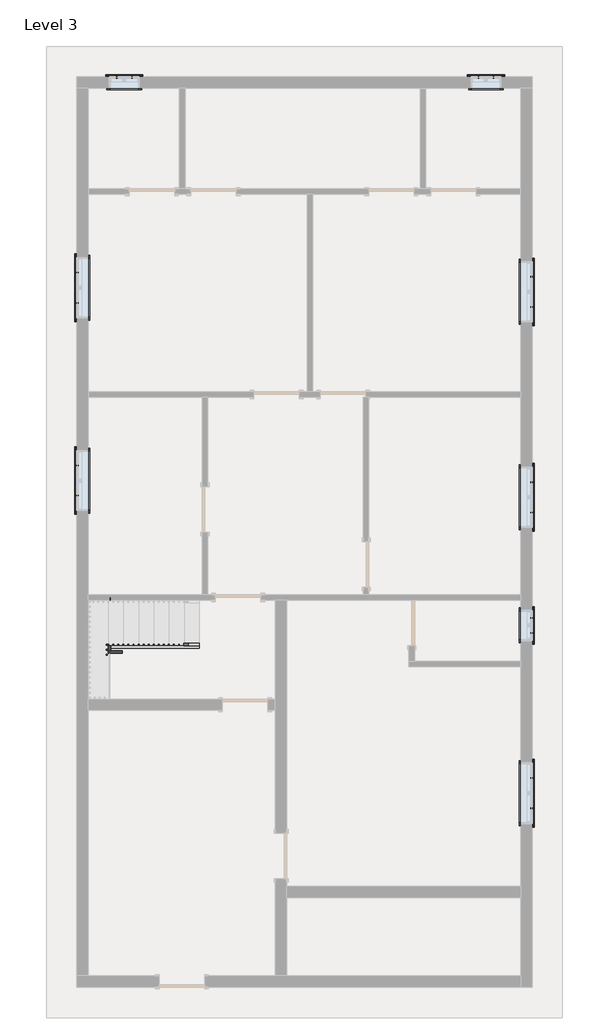
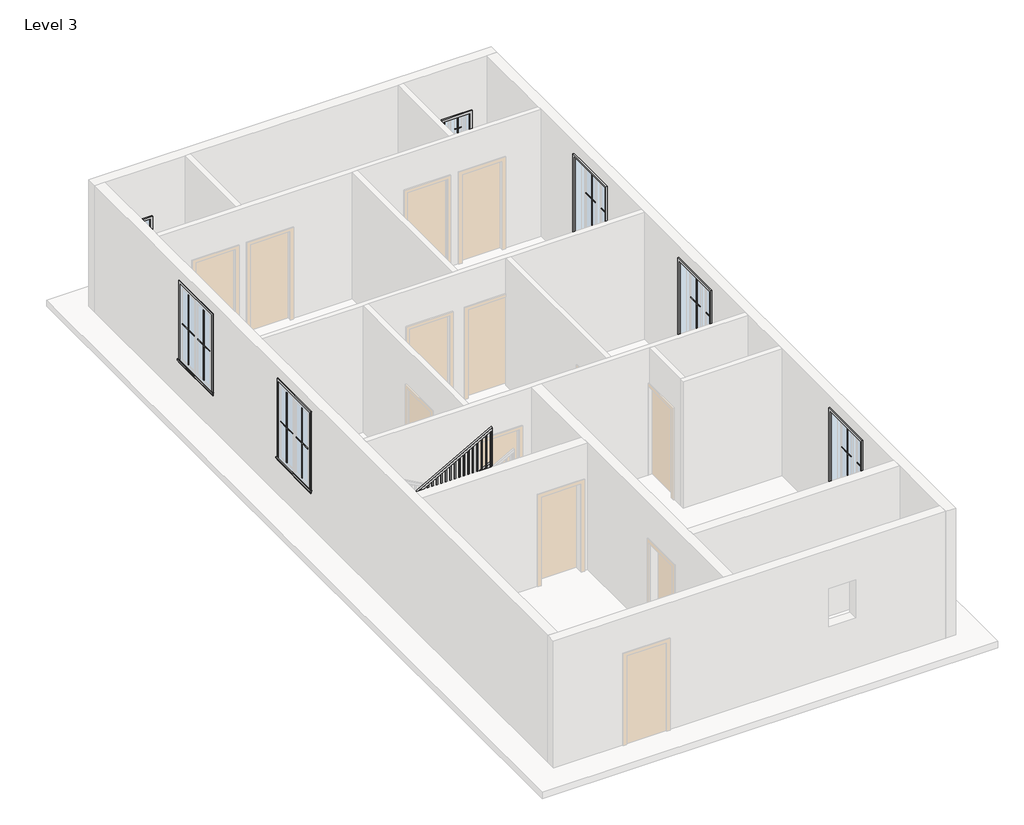
# One storey, part 3 of 3: 32 proxies, 6 members, 1 railing.
"""IFC4 building model written with IfcOpenShell, lengths in millimetres."""

from ifc_helpers import new_model, si_unit, frame, origin, place, context, project, spatial, polyline, outline, extrude, faceted_brep, transform, mapped, element, save
from components import muntin_pattern_2x2_muntin_pattern_2x2_2b4d9f72, muntin_pattern_2x2_muntin_pattern_2x2_ef995ed3, muntin_pattern_2x2_muntin_pattern_2x2_53152e2c, muntin_pattern_2x2_muntin_pattern_2x2_e8f3e573, trim_window_exterior_flat_with_sill_b7e4d11c, trim_window_exterior_flat_with_sill_a665a915, trim_window_interior_flat_picture_frame_936b8d2a, trim_window_interior_flat_picture_frame_d485c387

model = new_model("IFC4")

# Units and contexts
model_context = context("Model", 3, world=origin())
ifc_project = project(units=[si_unit("LENGTHUNIT", "METRE", prefix="MILLI")], contexts=[model_context])

# Site, building, storey
site = spatial("IfcSite", under=ifc_project)
building = spatial("IfcBuilding", under=site)
storey = spatial("IfcBuildingStorey", under=building, Name="Level 3", Elevation=6096.0)

# Proxies
placement = place(None, origin())
muntin_pattern_2x2_muntin_pattern_2x2_shape = muntin_pattern_2x2_muntin_pattern_2x2_2b4d9f72(model_context)
element("IfcBuildingElementProxy", 1, Name="Muntin Pattern_2x2 : Muntin Pattern_2x2", ObjectType="Muntin Pattern_2x2 : Muntin Pattern_2x2", at=placement, inside=storey, context=model_context, shape_type="MappedRepresentation", body=[
    mapped(muntin_pattern_2x2_muntin_pattern_2x2_shape, transform((1279.525, 5811.8375, 7080.25), x_axis=(0.0, 1.0, 0.0), y_axis=(-1.0, 0.0, 0.0), z_axis=(0.0, 0.0, 1.0))),
])
element("IfcBuildingElementProxy", 2, Name="Muntin Pattern_2x2 : Muntin Pattern_2x2", ObjectType="Muntin Pattern_2x2 : Muntin Pattern_2x2", at=placement, inside=storey, context=model_context, shape_type="MappedRepresentation", body=[
    mapped(muntin_pattern_2x2_muntin_pattern_2x2_shape, transform((1279.525, 9685.3375, 7080.25), x_axis=(0.0, 1.0, 0.0), y_axis=(-1.0, 0.0, 0.0), z_axis=(0.0, 0.0, 1.0))),
])
element("IfcBuildingElementProxy", 3, Name="Muntin Pattern_2x2 : Muntin Pattern_2x2", ObjectType="Muntin Pattern_2x2 : Muntin Pattern_2x2", at=placement, inside=storey, context=model_context, shape_type="MappedRepresentation", body=[
    mapped(muntin_pattern_2x2_muntin_pattern_2x2_shape, transform((10404.475, 10209.2125, 7080.25), x_axis=(0.0, -1.0, 0.0), y_axis=(1.0, 0.0, 0.0), z_axis=(0.0, 0.0, 1.0))),
])
element("IfcBuildingElementProxy", 4, Name="Muntin Pattern_2x2 : Muntin Pattern_2x2", ObjectType="Muntin Pattern_2x2 : Muntin Pattern_2x2", at=placement, inside=storey, context=model_context, shape_type="MappedRepresentation", body=[
    mapped(muntin_pattern_2x2_muntin_pattern_2x2_shape, transform((10404.475, 6081.7125, 7080.25), x_axis=(0.0, -1.0, 0.0), y_axis=(1.0, 0.0, 0.0), z_axis=(0.0, 0.0, 1.0))),
])
element("IfcBuildingElementProxy", 5, Name="Muntin Pattern_2x2 : Muntin Pattern_2x2", ObjectType="Muntin Pattern_2x2 : Muntin Pattern_2x2", at=placement, inside=storey, context=model_context, shape_type="MappedRepresentation", body=[
    mapped(muntin_pattern_2x2_muntin_pattern_2x2_shape, transform((10404.475, 138.1125, 7080.25), x_axis=(0.0, -1.0, 0.0), y_axis=(1.0, 0.0, 0.0), z_axis=(0.0, 0.0, 1.0))),
])
muntin_pattern_2x2_muntin_pattern_2x2_2_shape = muntin_pattern_2x2_muntin_pattern_2x2_ef995ed3(model_context)
element("IfcBuildingElementProxy", 6, Name="Muntin Pattern_2x2 : Muntin Pattern_2x2", ObjectType="Muntin Pattern_2x2 : Muntin Pattern_2x2", at=placement, inside=storey, context=model_context, shape_type="MappedRepresentation", body=[
    mapped(muntin_pattern_2x2_muntin_pattern_2x2_2_shape, transform((1279.525, 6418.2625, 7080.25), x_axis=(0.0, -1.0, 0.0), y_axis=(1.0, 0.0, 0.0), z_axis=(0.0, 0.0, 1.0))),
])
element("IfcBuildingElementProxy", 7, Name="Muntin Pattern_2x2 : Muntin Pattern_2x2", ObjectType="Muntin Pattern_2x2 : Muntin Pattern_2x2", at=placement, inside=storey, context=model_context, shape_type="MappedRepresentation", body=[
    mapped(muntin_pattern_2x2_muntin_pattern_2x2_2_shape, transform((1279.525, 10291.7625, 7080.25), x_axis=(0.0, -1.0, 0.0), y_axis=(1.0, 0.0, 0.0), z_axis=(0.0, 0.0, 1.0))),
])
element("IfcBuildingElementProxy", 8, Name="Muntin Pattern_2x2 : Muntin Pattern_2x2", ObjectType="Muntin Pattern_2x2 : Muntin Pattern_2x2", at=placement, inside=storey, context=model_context, shape_type="MappedRepresentation", body=[
    mapped(muntin_pattern_2x2_muntin_pattern_2x2_2_shape, transform((10404.475, 9602.7875, 7080.25), x_axis=(0.0, 1.0, 0.0), y_axis=(-1.0, 0.0, 0.0), z_axis=(0.0, 0.0, 1.0))),
])
element("IfcBuildingElementProxy", 9, Name="Muntin Pattern_2x2 : Muntin Pattern_2x2", ObjectType="Muntin Pattern_2x2 : Muntin Pattern_2x2", at=placement, inside=storey, context=model_context, shape_type="MappedRepresentation", body=[
    mapped(muntin_pattern_2x2_muntin_pattern_2x2_2_shape, transform((10404.475, 5475.2875, 7080.25), x_axis=(0.0, 1.0, 0.0), y_axis=(-1.0, 0.0, 0.0), z_axis=(0.0, 0.0, 1.0))),
])
element("IfcBuildingElementProxy", 10, Name="Muntin Pattern_2x2 : Muntin Pattern_2x2", ObjectType="Muntin Pattern_2x2 : Muntin Pattern_2x2", at=placement, inside=storey, context=model_context, shape_type="MappedRepresentation", body=[
    mapped(muntin_pattern_2x2_muntin_pattern_2x2_2_shape, transform((10404.475, -468.3125, 7080.25), x_axis=(0.0, 1.0, 0.0), y_axis=(-1.0, 0.0, 0.0), z_axis=(0.0, 0.0, 1.0))),
])
muntin_pattern_2x2_muntin_pattern_2x2_3_shape = muntin_pattern_2x2_muntin_pattern_2x2_53152e2c(model_context)
element("IfcBuildingElementProxy", 11, Name="Muntin Pattern_2x2 : Muntin Pattern_2x2", ObjectType="Muntin Pattern_2x2 : Muntin Pattern_2x2", at=placement, inside=storey, context=model_context, shape_type="MappedRepresentation", body=[
    mapped(muntin_pattern_2x2_muntin_pattern_2x2_3_shape, transform((10404.475, 3357.5625, 7080.25), x_axis=(0.0, -1.0, 0.0), y_axis=(1.0, 0.0, 0.0), z_axis=(0.0, 0.0, 1.0))),
])
element("IfcBuildingElementProxy", 12, Name="Muntin Pattern_2x2 : Muntin Pattern_2x2", ObjectType="Muntin Pattern_2x2 : Muntin Pattern_2x2", at=placement, inside=storey, context=model_context, shape_type="MappedRepresentation", body=[
    mapped(muntin_pattern_2x2_muntin_pattern_2x2_3_shape, transform((9336.0875, 14214.475, 7080.25), x_axis=(1.0, 0.0, 0.0), y_axis=(0.0, 1.0, 0.0), z_axis=(0.0, 0.0, 1.0))),
])
element("IfcBuildingElementProxy", 13, Name="Muntin Pattern_2x2 : Muntin Pattern_2x2", ObjectType="Muntin Pattern_2x2 : Muntin Pattern_2x2", at=placement, inside=storey, context=model_context, shape_type="MappedRepresentation", body=[
    mapped(muntin_pattern_2x2_muntin_pattern_2x2_3_shape, transform((2071.6875, 14214.475, 7080.25), x_axis=(1.0, 0.0, 0.0), y_axis=(0.0, 1.0, 0.0), z_axis=(0.0, 0.0, 1.0))),
])
muntin_pattern_2x2_muntin_pattern_2x2_4_shape = muntin_pattern_2x2_muntin_pattern_2x2_e8f3e573(model_context)
element("IfcBuildingElementProxy", 14, Name="Muntin Pattern_2x2 : Muntin Pattern_2x2", ObjectType="Muntin Pattern_2x2 : Muntin Pattern_2x2", at=placement, inside=storey, context=model_context, shape_type="MappedRepresentation", body=[
    mapped(muntin_pattern_2x2_muntin_pattern_2x2_4_shape, transform((10404.475, 3055.9375, 7080.25), x_axis=(0.0, 1.0, 0.0), y_axis=(-1.0, 0.0, 0.0), z_axis=(0.0, 0.0, 1.0))),
])
element("IfcBuildingElementProxy", 15, Name="Muntin Pattern_2x2 : Muntin Pattern_2x2", ObjectType="Muntin Pattern_2x2 : Muntin Pattern_2x2", at=placement, inside=storey, context=model_context, shape_type="MappedRepresentation", body=[
    mapped(muntin_pattern_2x2_muntin_pattern_2x2_4_shape, transform((9637.7125, 14214.475, 7080.25), x_axis=(-1.0, 0.0, 0.0), y_axis=(0.0, -1.0, 0.0), z_axis=(0.0, 0.0, 1.0))),
])
element("IfcBuildingElementProxy", 16, Name="Muntin Pattern_2x2 : Muntin Pattern_2x2", ObjectType="Muntin Pattern_2x2 : Muntin Pattern_2x2", at=placement, inside=storey, context=model_context, shape_type="MappedRepresentation", body=[
    mapped(muntin_pattern_2x2_muntin_pattern_2x2_4_shape, transform((2373.3125, 14214.475, 7080.25), x_axis=(-1.0, 0.0, 0.0), y_axis=(0.0, -1.0, 0.0), z_axis=(0.0, 0.0, 1.0))),
])
trim_window_exterior_flat_with_sill_shape = trim_window_exterior_flat_with_sill_b7e4d11c(model_context)
element("IfcBuildingElementProxy", 17, Name="Trim-Window-Exterior-Flat : with Sill", ObjectType="Trim-Window-Exterior-Flat : with Sill", at=placement, inside=storey, context=model_context, shape_type="MappedRepresentation", body=[
    mapped(trim_window_exterior_flat_with_sill_shape, transform((1270.0, 6115.05, 8839.2), x_axis=(0.0, -1.0, 0.0), y_axis=(0.0, 0.0, 1.0), z_axis=(-1.0, 0.0, 0.0))),
])
element("IfcBuildingElementProxy", 18, Name="Trim-Window-Exterior-Flat : with Sill", ObjectType="Trim-Window-Exterior-Flat : with Sill", at=placement, inside=storey, context=model_context, shape_type="MappedRepresentation", body=[
    mapped(trim_window_exterior_flat_with_sill_shape, transform((1270.0, 9988.55, 8839.2), x_axis=(0.0, -1.0, 0.0), y_axis=(0.0, 0.0, 1.0), z_axis=(-1.0, 0.0, 0.0))),
])
element("IfcBuildingElementProxy", 19, Name="Trim-Window-Exterior-Flat : with Sill", ObjectType="Trim-Window-Exterior-Flat : with Sill", at=placement, inside=storey, context=model_context, shape_type="MappedRepresentation", body=[
    mapped(trim_window_exterior_flat_with_sill_shape, transform((10414.0, 9906.0, 8839.2), x_axis=(0.0, 1.0, 0.0), y_axis=(0.0, 0.0, 1.0), z_axis=(1.0, 0.0, 0.0))),
])
element("IfcBuildingElementProxy", 20, Name="Trim-Window-Exterior-Flat : with Sill", ObjectType="Trim-Window-Exterior-Flat : with Sill", at=placement, inside=storey, context=model_context, shape_type="MappedRepresentation", body=[
    mapped(trim_window_exterior_flat_with_sill_shape, transform((10414.0, 5778.5, 8839.2), x_axis=(0.0, 1.0, 0.0), y_axis=(0.0, 0.0, 1.0), z_axis=(1.0, 0.0, 0.0))),
])
element("IfcBuildingElementProxy", 21, Name="Trim-Window-Exterior-Flat : with Sill", ObjectType="Trim-Window-Exterior-Flat : with Sill", at=placement, inside=storey, context=model_context, shape_type="MappedRepresentation", body=[
    mapped(trim_window_exterior_flat_with_sill_shape, transform((10414.0, -165.1, 8839.2), x_axis=(0.0, 1.0, 0.0), y_axis=(0.0, 0.0, 1.0), z_axis=(1.0, 0.0, 0.0))),
])
trim_window_exterior_flat_with_sill_2_shape = trim_window_exterior_flat_with_sill_a665a915(model_context)
element("IfcBuildingElementProxy", 22, Name="Trim-Window-Exterior-Flat : with Sill", ObjectType="Trim-Window-Exterior-Flat : with Sill", at=placement, inside=storey, context=model_context, shape_type="MappedRepresentation", body=[
    mapped(trim_window_exterior_flat_with_sill_2_shape, transform((10414.0, 3206.75, 7924.8), x_axis=(0.0, 1.0, 0.0), y_axis=(0.0, 0.0, 1.0), z_axis=(1.0, 0.0, 0.0))),
])
element("IfcBuildingElementProxy", 23, Name="Trim-Window-Exterior-Flat : with Sill", ObjectType="Trim-Window-Exterior-Flat : with Sill", at=placement, inside=storey, context=model_context, shape_type="MappedRepresentation", body=[
    mapped(trim_window_exterior_flat_with_sill_2_shape, transform((9486.9, 14224.0, 7924.8), x_axis=(-1.0, 0.0, 0.0), y_axis=(0.0, 0.0, 1.0), z_axis=(0.0, 1.0, 0.0))),
])
element("IfcBuildingElementProxy", 24, Name="Trim-Window-Exterior-Flat : with Sill", ObjectType="Trim-Window-Exterior-Flat : with Sill", at=placement, inside=storey, context=model_context, shape_type="MappedRepresentation", body=[
    mapped(trim_window_exterior_flat_with_sill_2_shape, transform((2222.5, 14224.0, 7924.8), x_axis=(-1.0, 0.0, 0.0), y_axis=(0.0, 0.0, 1.0), z_axis=(0.0, 1.0, 0.0))),
])
trim_window_interior_flat_picture_frame_shape = trim_window_interior_flat_picture_frame_936b8d2a(model_context)
element("IfcBuildingElementProxy", 25, Name="Trim-Window-Interior-Flat : Picture Frame", ObjectType="Trim-Window-Interior-Flat : Picture Frame", at=placement, inside=storey, context=model_context, shape_type="MappedRepresentation", body=[
    mapped(trim_window_interior_flat_picture_frame_shape, transform((1498.6, 6115.05, 8839.2), x_axis=(0.0, 1.0, 0.0), y_axis=(0.0, 0.0, 1.0), z_axis=(1.0, 0.0, 0.0))),
])
element("IfcBuildingElementProxy", 26, Name="Trim-Window-Interior-Flat : Picture Frame", ObjectType="Trim-Window-Interior-Flat : Picture Frame", at=placement, inside=storey, context=model_context, shape_type="MappedRepresentation", body=[
    mapped(trim_window_interior_flat_picture_frame_shape, transform((1498.6, 9988.55, 8839.2), x_axis=(0.0, 1.0, 0.0), y_axis=(0.0, 0.0, 1.0), z_axis=(1.0, 0.0, 0.0))),
])
element("IfcBuildingElementProxy", 27, Name="Trim-Window-Interior-Flat : Picture Frame", ObjectType="Trim-Window-Interior-Flat : Picture Frame", at=placement, inside=storey, context=model_context, shape_type="MappedRepresentation", body=[
    mapped(trim_window_interior_flat_picture_frame_shape, transform((10185.4, 9906.0, 8839.2), x_axis=(0.0, -1.0, 0.0), y_axis=(0.0, 0.0, 1.0), z_axis=(-1.0, 0.0, 0.0))),
])
element("IfcBuildingElementProxy", 28, Name="Trim-Window-Interior-Flat : Picture Frame", ObjectType="Trim-Window-Interior-Flat : Picture Frame", at=placement, inside=storey, context=model_context, shape_type="MappedRepresentation", body=[
    mapped(trim_window_interior_flat_picture_frame_shape, transform((10185.4, 5778.5, 8839.2), x_axis=(0.0, -1.0, 0.0), y_axis=(0.0, 0.0, 1.0), z_axis=(-1.0, 0.0, 0.0))),
])
element("IfcBuildingElementProxy", 29, Name="Trim-Window-Interior-Flat : Picture Frame", ObjectType="Trim-Window-Interior-Flat : Picture Frame", at=placement, inside=storey, context=model_context, shape_type="MappedRepresentation", body=[
    mapped(trim_window_interior_flat_picture_frame_shape, transform((10185.4, -165.1, 8839.2), x_axis=(0.0, -1.0, 0.0), y_axis=(0.0, 0.0, 1.0), z_axis=(-1.0, 0.0, 0.0))),
])
trim_window_interior_flat_picture_frame_2_shape = trim_window_interior_flat_picture_frame_d485c387(model_context)
element("IfcBuildingElementProxy", 30, Name="Trim-Window-Interior-Flat : Picture Frame", ObjectType="Trim-Window-Interior-Flat : Picture Frame", at=placement, inside=storey, context=model_context, shape_type="MappedRepresentation", body=[
    mapped(trim_window_interior_flat_picture_frame_2_shape, transform((10185.4, 3206.75, 7924.8), x_axis=(0.0, -1.0, 0.0), y_axis=(0.0, 0.0, 1.0), z_axis=(-1.0, 0.0, 0.0))),
])
element("IfcBuildingElementProxy", 31, Name="Trim-Window-Interior-Flat : Picture Frame", ObjectType="Trim-Window-Interior-Flat : Picture Frame", at=placement, inside=storey, context=model_context, shape_type="MappedRepresentation", body=[
    mapped(trim_window_interior_flat_picture_frame_2_shape, transform((9486.9, 13995.4, 7924.8), x_axis=(1.0, 0.0, 0.0), y_axis=(0.0, 0.0, 1.0), z_axis=(0.0, -1.0, 0.0))),
])
element("IfcBuildingElementProxy", 32, Name="Trim-Window-Interior-Flat : Picture Frame", ObjectType="Trim-Window-Interior-Flat : Picture Frame", at=placement, inside=storey, context=model_context, shape_type="MappedRepresentation", body=[
    mapped(trim_window_interior_flat_picture_frame_2_shape, transform((2222.5, 13995.4, 7924.8), x_axis=(1.0, 0.0, 0.0), y_axis=(0.0, 0.0, 1.0), z_axis=(0.0, -1.0, 0.0))),
])

# Members
element("IfcMember", 33, ObjectType="Stringer - 2\" Width", at=placement, inside=storey, context=model_context, shape_type="SweptSolid", body=[
    extrude(outline(polyline([(6096.0, 3727.9146873), (6303.5983948, 3727.9146873), (7291.3761726, 1949.9146873), (6942.6974984, 1949.9146873), (6096.0, 3473.9701845), (6096.0, 3727.9146873)])), frame((0.0, 2743.2, 0.0), z_axis=(0.0, 1.0, 0.0), x_axis=(0.0, 0.0, 1.0)), (0.0, 0.0, 1.0), 50.8),
])
element("IfcMember", 34, ObjectType="Stringer - 2\" Width", at=placement, inside=storey, context=model_context, shape_type="SweptSolid", body=[
    extrude(outline(polyline([(1899.1146873, 2794.0), (1949.9146873, 2794.0), (1949.9146873, 2692.4), (1899.1146873, 2692.4), (1899.1146873, 2794.0)])), frame((0.0, 0.0, 7052.7333333), z_axis=(0.0, 0.0, 1.0), x_axis=(1.0, 0.0, 0.0)), (0.0, 0.0, 1.0), 304.8),
])
element("IfcMember", 35, ObjectType="Stringer - 2\" Width", at=placement, inside=storey, context=model_context, shape_type="SweptSolid", body=[
    extrude(outline(polyline([(7488.9317281, 1899.1146873), (7140.253054, 1899.1146873), (8156.253054, 3727.9146873), (8504.9317281, 3727.9146873), (7488.9317281, 1899.1146873)])), frame((0.0, 2641.6, 0.0), z_axis=(0.0, 1.0, 0.0), x_axis=(0.0, 0.0, 1.0)), (0.0, 0.0, 1.0), 50.8),
])
element("IfcMember", 36, ObjectType="Stringer - 2\" Width", at=placement, inside=storey, context=model_context, shape_type="SweptSolid", body=[
    extrude(outline(polyline([(6096.0, 3727.9146873), (6303.5983948, 3727.9146873), (7357.5333333, 1830.8317979), (7357.5333333, 1498.6), (7193.4278803, 1498.6), (6096.0, 3473.9701845), (6096.0, 3727.9146873)])), frame((0.0, 3708.4, 0.0), z_axis=(0.0, 1.0, 0.0), x_axis=(0.0, 0.0, 1.0)), (0.0, 0.0, 1.0), 50.8),
])
element("IfcMember", 37, ObjectType="Stringer - 2\" Width", at=placement, inside=storey, context=model_context, shape_type="SweptSolid", body=[
    extrude(outline(polyline([(1447.8, 3759.2), (1498.6, 3759.2), (1498.6, 1727.2), (1447.8, 1727.2), (1447.8, 3759.2)])), frame((0.0, 0.0, 7052.7333333), z_axis=(0.0, 0.0, 1.0), x_axis=(1.0, 0.0, 0.0)), (0.0, 0.0, 1.0), 304.8),
])
element("IfcMember", 38, ObjectType="Stringer - 2\" Width", at=placement, inside=storey, context=model_context, shape_type="SweptSolid", body=[
    extrude(outline(polyline([(7238.2013463, 1447.8), (7052.7333333, 1447.8), (7052.7333333, 1741.5791901), (8156.253054, 3727.9146873), (8504.9317281, 3727.9146873), (7238.2013463, 1447.8)])), frame((0.0, 1676.4, 0.0), z_axis=(0.0, 1.0, 0.0), x_axis=(0.0, 0.0, 1.0)), (0.0, 0.0, 1.0), 50.8),
])

# Railing
element("IfcRailing", 39, ObjectType="Handrail - Rectangular", at=placement, inside=storey, context=model_context, shape_type="SolidModel", body=[
    faceted_brep([(3727.9146873, 2794.0, 7179.7333333), (3727.9146873, 2794.0, 7121.620221), (3727.9146873, 2844.8, 7121.620221), (3727.9146873, 2844.8, 7179.7333333), (1975.3146873, 2794.0, 8153.4), (1924.5146873, 2794.0, 8123.5091099), (1924.5146873, 2844.8, 8123.5091099), (1975.3146873, 2844.8, 8153.4), (1975.3146873, 2794.0, 8195.7333333), (1924.5146873, 2794.0, 8144.9333333), (1924.5146873, 2844.8, 8144.9333333), (1975.3146873, 2844.8, 8195.7333333), (1899.1146873, 2794.0, 8195.7333333), (1899.1146873, 2794.0, 8144.9333333), (1848.3146873, 2844.8, 8144.9333333), (1848.3146873, 2844.8, 8195.7333333), (1899.1146873, 2717.8, 8195.7333333), (1899.1146873, 2667.0, 8144.9333333), (1848.3146873, 2667.0, 8144.9333333), (1848.3146873, 2717.8, 8195.7333333), (1899.1146873, 2717.8, 8407.4), (1899.1146873, 2667.0, 8356.6), (1848.3146873, 2667.0, 8356.6), (1848.3146873, 2717.8, 8407.4), (1899.1146873, 2641.6, 8407.4), (1899.1146873, 2641.6, 8356.6), (1848.3146873, 2590.8, 8356.6), (1848.3146873, 2590.8, 8407.4), (1975.3146873, 2641.6, 8407.4), (1988.4782895, 2641.6, 8356.6), (1988.4782895, 2590.8, 8356.6), (1975.3146873, 2590.8, 8407.4), (3727.9146873, 2641.6, 9381.0666667), (3727.9146873, 2590.8, 9381.0666667), (3727.9146873, 2590.8, 9322.9535543), (3727.9146873, 2641.6, 9322.9535543)], [[[0, 1, 2, 3]], [[1, 0, 4, 5]], [[2, 1, 5, 6]], [[3, 2, 6, 7]], [[0, 3, 7, 4]], [[5, 4, 8, 9]], [[6, 5, 9, 10]], [[7, 6, 10, 11]], [[4, 7, 11, 8]], [[9, 8, 12, 13]], [[10, 9, 13, 14]], [[11, 10, 14, 15]], [[8, 11, 15, 12]], [[13, 12, 16, 17]], [[14, 13, 17, 18]], [[15, 14, 18, 19]], [[12, 15, 19, 16]], [[17, 16, 20, 21]], [[18, 17, 21, 22]], [[19, 18, 22, 23]], [[16, 19, 23, 20]], [[21, 20, 24, 25]], [[22, 21, 25, 26]], [[23, 22, 26, 27]], [[20, 23, 27, 24]], [[25, 24, 28, 29]], [[26, 25, 29, 30]], [[27, 26, 30, 31]], [[24, 27, 31, 28]], [[32, 33, 34, 35]], [[29, 28, 32, 35]], [[30, 29, 35, 34]], [[31, 30, 34, 33]], [[28, 31, 33, 32]]]),
    extrude(outline(polyline([(9303.5507765, 3692.9896873), (8297.3333333, 3692.9896873), (8297.3333333, 3712.0396873), (9314.1341099, 3712.0396873), (9303.5507765, 3692.9896873)])), frame((0.0, 2606.675, 0.0), z_axis=(0.0, 1.0, 0.0), x_axis=(0.0, 0.0, 1.0)), (0.0, 0.0, 1.0), 19.05),
    extrude(outline(polyline([(9247.1063321, 3591.3896873), (8297.3333333, 3591.3896873), (8297.3333333, 3610.4396873), (9257.6896654, 3610.4396873), (9247.1063321, 3591.3896873)])), frame((0.0, 2606.675, 0.0), z_axis=(0.0, 1.0, 0.0), x_axis=(0.0, 0.0, 1.0)), (0.0, 0.0, 1.0), 19.05),
    extrude(outline(polyline([(9190.6618876, 3489.7896873), (8297.3333333, 3489.7896873), (8297.3333333, 3508.8396873), (9201.245221, 3508.8396873), (9190.6618876, 3489.7896873)])), frame((0.0, 2606.675, 0.0), z_axis=(0.0, 1.0, 0.0), x_axis=(0.0, 0.0, 1.0)), (0.0, 0.0, 1.0), 19.05),
    extrude(outline(polyline([(9134.2174432, 3388.1896873), (8128.0, 3388.1896873), (8128.0, 3407.2396873), (9144.8007765, 3407.2396873), (9134.2174432, 3388.1896873)])), frame((0.0, 2606.675, 0.0), z_axis=(0.0, 1.0, 0.0), x_axis=(0.0, 0.0, 1.0)), (0.0, 0.0, 1.0), 19.05),
    extrude(outline(polyline([(9077.7729988, 3286.5896873), (8128.0, 3286.5896873), (8128.0, 3305.6396873), (9088.3563321, 3305.6396873), (9077.7729988, 3286.5896873)])), frame((0.0, 2606.675, 0.0), z_axis=(0.0, 1.0, 0.0), x_axis=(0.0, 0.0, 1.0)), (0.0, 0.0, 1.0), 19.05),
    extrude(outline(polyline([(9021.3285543, 3184.9896873), (8128.0, 3184.9896873), (8128.0, 3204.0396873), (9031.9118876, 3204.0396873), (9021.3285543, 3184.9896873)])), frame((0.0, 2606.675, 0.0), z_axis=(0.0, 1.0, 0.0), x_axis=(0.0, 0.0, 1.0)), (0.0, 0.0, 1.0), 19.05),
    extrude(outline(polyline([(8964.8841099, 3083.3896873), (7958.6666667, 3083.3896873), (7958.6666667, 3102.4396873), (8975.4674432, 3102.4396873), (8964.8841099, 3083.3896873)])), frame((0.0, 2606.675, 0.0), z_axis=(0.0, 1.0, 0.0), x_axis=(0.0, 0.0, 1.0)), (0.0, 0.0, 1.0), 19.05),
    extrude(outline(polyline([(8908.4396654, 2981.7896873), (7958.6666667, 2981.7896873), (7958.6666667, 3000.8396873), (8919.0229988, 3000.8396873), (8908.4396654, 2981.7896873)])), frame((0.0, 2606.675, 0.0), z_axis=(0.0, 1.0, 0.0), x_axis=(0.0, 0.0, 1.0)), (0.0, 0.0, 1.0), 19.05),
    extrude(outline(polyline([(8851.995221, 2880.1896873), (7958.6666667, 2880.1896873), (7958.6666667, 2899.2396873), (8862.5785543, 2899.2396873), (8851.995221, 2880.1896873)])), frame((0.0, 2606.675, 0.0), z_axis=(0.0, 1.0, 0.0), x_axis=(0.0, 0.0, 1.0)), (0.0, 0.0, 1.0), 19.05),
    extrude(outline(polyline([(8795.5507765, 2778.5896873), (7789.3333333, 2778.5896873), (7789.3333333, 2797.6396873), (8806.1341099, 2797.6396873), (8795.5507765, 2778.5896873)])), frame((0.0, 2606.675, 0.0), z_axis=(0.0, 1.0, 0.0), x_axis=(0.0, 0.0, 1.0)), (0.0, 0.0, 1.0), 19.05),
    extrude(outline(polyline([(8739.1063321, 2676.9896873), (7789.3333333, 2676.9896873), (7789.3333333, 2696.0396873), (8749.6896654, 2696.0396873), (8739.1063321, 2676.9896873)])), frame((0.0, 2606.675, 0.0), z_axis=(0.0, 1.0, 0.0), x_axis=(0.0, 0.0, 1.0)), (0.0, 0.0, 1.0), 19.05),
    extrude(outline(polyline([(8682.6618876, 2575.3896873), (7789.3333333, 2575.3896873), (7789.3333333, 2594.4396873), (8693.245221, 2594.4396873), (8682.6618876, 2575.3896873)])), frame((0.0, 2606.675, 0.0), z_axis=(0.0, 1.0, 0.0), x_axis=(0.0, 0.0, 1.0)), (0.0, 0.0, 1.0), 19.05),
    extrude(outline(polyline([(8626.2174432, 2473.7896873), (7620.0, 2473.7896873), (7620.0, 2492.8396873), (8636.8007765, 2492.8396873), (8626.2174432, 2473.7896873)])), frame((0.0, 2606.675, 0.0), z_axis=(0.0, 1.0, 0.0), x_axis=(0.0, 0.0, 1.0)), (0.0, 0.0, 1.0), 19.05),
    extrude(outline(polyline([(8569.7729988, 2372.1896873), (7620.0, 2372.1896873), (7620.0, 2391.2396873), (8580.3563321, 2391.2396873), (8569.7729988, 2372.1896873)])), frame((0.0, 2606.675, 0.0), z_axis=(0.0, 1.0, 0.0), x_axis=(0.0, 0.0, 1.0)), (0.0, 0.0, 1.0), 19.05),
    extrude(outline(polyline([(8513.3285543, 2270.5896873), (7620.0, 2270.5896873), (7620.0, 2289.6396873), (8523.9118876, 2289.6396873), (8513.3285543, 2270.5896873)])), frame((0.0, 2606.675, 0.0), z_axis=(0.0, 1.0, 0.0), x_axis=(0.0, 0.0, 1.0)), (0.0, 0.0, 1.0), 19.05),
    extrude(outline(polyline([(8456.8841099, 2168.9896873), (7450.6666667, 2168.9896873), (7450.6666667, 2188.0396873), (8467.4674432, 2188.0396873), (8456.8841099, 2168.9896873)])), frame((0.0, 2606.675, 0.0), z_axis=(0.0, 1.0, 0.0), x_axis=(0.0, 0.0, 1.0)), (0.0, 0.0, 1.0), 19.05),
    extrude(outline(polyline([(8400.4396654, 2067.3896873), (7450.6666667, 2067.3896873), (7450.6666667, 2086.4396873), (8411.0229988, 2086.4396873), (8400.4396654, 2067.3896873)])), frame((0.0, 2606.675, 0.0), z_axis=(0.0, 1.0, 0.0), x_axis=(0.0, 0.0, 1.0)), (0.0, 0.0, 1.0), 19.05),
    extrude(outline(polyline([(8343.995221, 1965.7896873), (7450.6666667, 1965.7896873), (7450.6666667, 1984.8396873), (8354.5785543, 1984.8396873), (8343.995221, 1965.7896873)])), frame((0.0, 2606.675, 0.0), z_axis=(0.0, 1.0, 0.0), x_axis=(0.0, 0.0, 1.0)), (0.0, 0.0, 1.0), 19.05),
    extrude(outline(polyline([(1883.2396873, 2727.325), (1883.2396873, 2708.275), (1864.1896873, 2708.275), (1864.1896873, 2727.325), (1883.2396873, 2727.325)])), frame((0.0, 0.0, 7281.3333333), z_axis=(0.0, 0.0, 1.0), x_axis=(1.0, 0.0, 0.0)), (0.0, 0.0, 1.0), 863.6),
    extrude(outline(polyline([(1908.6396873, 2809.875), (1889.5896873, 2809.875), (1889.5896873, 2828.925), (1908.6396873, 2828.925), (1908.6396873, 2809.875)])), frame((0.0, 0.0, 7281.3333333), z_axis=(0.0, 0.0, 1.0), x_axis=(1.0, 0.0, 0.0)), (0.0, 0.0, 1.0), 863.6),
    extrude(outline(polyline([(8086.4674432, 1991.1896873), (7112.0, 1991.1896873), (7112.0, 2010.2396873), (8075.8841099, 2010.2396873), (8086.4674432, 1991.1896873)])), frame((0.0, 2809.875, 0.0), z_axis=(0.0, 1.0, 0.0), x_axis=(0.0, 0.0, 1.0)), (0.0, 0.0, 1.0), 19.05),
    extrude(outline(polyline([(8030.0229988, 2092.7896873), (7112.0, 2092.7896873), (7112.0, 2111.8396873), (8019.4396654, 2111.8396873), (8030.0229988, 2092.7896873)])), frame((0.0, 2809.875, 0.0), z_axis=(0.0, 1.0, 0.0), x_axis=(0.0, 0.0, 1.0)), (0.0, 0.0, 1.0), 19.05),
    extrude(outline(polyline([(7973.5785543, 2194.3896873), (7112.0, 2194.3896873), (7112.0, 2213.4396873), (7962.995221, 2213.4396873), (7973.5785543, 2194.3896873)])), frame((0.0, 2809.875, 0.0), z_axis=(0.0, 1.0, 0.0), x_axis=(0.0, 0.0, 1.0)), (0.0, 0.0, 1.0), 19.05),
    extrude(outline(polyline([(7917.1341099, 2295.9896873), (6942.6666667, 2295.9896873), (6942.6666667, 2315.0396873), (7906.5507765, 2315.0396873), (7917.1341099, 2295.9896873)])), frame((0.0, 2809.875, 0.0), z_axis=(0.0, 1.0, 0.0), x_axis=(0.0, 0.0, 1.0)), (0.0, 0.0, 1.0), 19.05),
    extrude(outline(polyline([(7860.6896654, 2397.5896873), (6942.6666667, 2397.5896873), (6942.6666667, 2416.6396873), (7850.1063321, 2416.6396873), (7860.6896654, 2397.5896873)])), frame((0.0, 2809.875, 0.0), z_axis=(0.0, 1.0, 0.0), x_axis=(0.0, 0.0, 1.0)), (0.0, 0.0, 1.0), 19.05),
    extrude(outline(polyline([(7804.245221, 2499.1896873), (6942.6666667, 2499.1896873), (6942.6666667, 2518.2396873), (7793.6618876, 2518.2396873), (7804.245221, 2499.1896873)])), frame((0.0, 2809.875, 0.0), z_axis=(0.0, 1.0, 0.0), x_axis=(0.0, 0.0, 1.0)), (0.0, 0.0, 1.0), 19.05),
    extrude(outline(polyline([(7747.8007765, 2600.7896873), (6773.3333333, 2600.7896873), (6773.3333333, 2619.8396873), (7737.2174432, 2619.8396873), (7747.8007765, 2600.7896873)])), frame((0.0, 2809.875, 0.0), z_axis=(0.0, 1.0, 0.0), x_axis=(0.0, 0.0, 1.0)), (0.0, 0.0, 1.0), 19.05),
    extrude(outline(polyline([(7691.3563321, 2702.3896873), (6773.3333333, 2702.3896873), (6773.3333333, 2721.4396873), (7680.7729988, 2721.4396873), (7691.3563321, 2702.3896873)])), frame((0.0, 2809.875, 0.0), z_axis=(0.0, 1.0, 0.0), x_axis=(0.0, 0.0, 1.0)), (0.0, 0.0, 1.0), 19.05),
    extrude(outline(polyline([(7634.9118876, 2803.9896873), (6773.3333333, 2803.9896873), (6773.3333333, 2823.0396873), (7624.3285543, 2823.0396873), (7634.9118876, 2803.9896873)])), frame((0.0, 2809.875, 0.0), z_axis=(0.0, 1.0, 0.0), x_axis=(0.0, 0.0, 1.0)), (0.0, 0.0, 1.0), 19.05),
    extrude(outline(polyline([(7578.4674432, 2905.5896873), (6604.0, 2905.5896873), (6604.0, 2924.6396873), (7567.8841099, 2924.6396873), (7578.4674432, 2905.5896873)])), frame((0.0, 2809.875, 0.0), z_axis=(0.0, 1.0, 0.0), x_axis=(0.0, 0.0, 1.0)), (0.0, 0.0, 1.0), 19.05),
    extrude(outline(polyline([(7522.0229988, 3007.1896873), (6604.0, 3007.1896873), (6604.0, 3026.2396873), (7511.4396654, 3026.2396873), (7522.0229988, 3007.1896873)])), frame((0.0, 2809.875, 0.0), z_axis=(0.0, 1.0, 0.0), x_axis=(0.0, 0.0, 1.0)), (0.0, 0.0, 1.0), 19.05),
    extrude(outline(polyline([(7465.5785543, 3108.7896873), (6604.0, 3108.7896873), (6604.0, 3127.8396873), (7454.995221, 3127.8396873), (7465.5785543, 3108.7896873)])), frame((0.0, 2809.875, 0.0), z_axis=(0.0, 1.0, 0.0), x_axis=(0.0, 0.0, 1.0)), (0.0, 0.0, 1.0), 19.05),
    extrude(outline(polyline([(7409.1341099, 3210.3896873), (6434.6666667, 3210.3896873), (6434.6666667, 3229.4396873), (7398.5507765, 3229.4396873), (7409.1341099, 3210.3896873)])), frame((0.0, 2809.875, 0.0), z_axis=(0.0, 1.0, 0.0), x_axis=(0.0, 0.0, 1.0)), (0.0, 0.0, 1.0), 19.05),
    extrude(outline(polyline([(7352.6896654, 3311.9896873), (6434.6666667, 3311.9896873), (6434.6666667, 3331.0396873), (7342.1063321, 3331.0396873), (7352.6896654, 3311.9896873)])), frame((0.0, 2809.875, 0.0), z_axis=(0.0, 1.0, 0.0), x_axis=(0.0, 0.0, 1.0)), (0.0, 0.0, 1.0), 19.05),
    extrude(outline(polyline([(7296.245221, 3413.5896873), (6434.6666667, 3413.5896873), (6434.6666667, 3432.6396873), (7285.6618876, 3432.6396873), (7296.245221, 3413.5896873)])), frame((0.0, 2809.875, 0.0), z_axis=(0.0, 1.0, 0.0), x_axis=(0.0, 0.0, 1.0)), (0.0, 0.0, 1.0), 19.05),
    extrude(outline(polyline([(7239.8007765, 3515.1896873), (6265.3333333, 3515.1896873), (6265.3333333, 3534.2396873), (7229.2174432, 3534.2396873), (7239.8007765, 3515.1896873)])), frame((0.0, 2809.875, 0.0), z_axis=(0.0, 1.0, 0.0), x_axis=(0.0, 0.0, 1.0)), (0.0, 0.0, 1.0), 19.05),
    extrude(outline(polyline([(7183.3563321, 3616.7896873), (6265.3333333, 3616.7896873), (6265.3333333, 3635.8396873), (7172.7729988, 3635.8396873), (7183.3563321, 3616.7896873)])), frame((0.0, 2809.875, 0.0), z_axis=(0.0, 1.0, 0.0), x_axis=(0.0, 0.0, 1.0)), (0.0, 0.0, 1.0), 19.05),
    extrude(outline(polyline([(1883.2396873, 2625.725), (1883.2396873, 2606.675), (1864.1896873, 2606.675), (1864.1896873, 2625.725), (1883.2396873, 2625.725)])), frame((0.0, 0.0, 7281.3333333), z_axis=(0.0, 0.0, 1.0), x_axis=(1.0, 0.0, 0.0)), (0.0, 0.0, 1.0), 1075.2666667),
    extrude(outline(polyline([(1883.2396873, 2809.875), (1864.1896873, 2809.875), (1864.1896873, 2828.925), (1883.2396873, 2828.925), (1883.2396873, 2809.875)])), frame((0.0, 0.0, 7281.3333333), z_axis=(0.0, 0.0, 1.0), x_axis=(1.0, 0.0, 0.0)), (0.0, 0.0, 1.0), 863.6),
    extrude(outline(polyline([(9312.370221, 3708.8646873), (8297.3333333, 3708.8646873), (8297.3333333, 3727.9146873), (9322.9535543, 3727.9146873), (9312.370221, 3708.8646873)])), frame((0.0, 2606.675, 0.0), z_axis=(0.0, 1.0, 0.0), x_axis=(0.0, 0.0, 1.0)), (0.0, 0.0, 1.0), 19.05),
    extrude(outline(polyline([(7132.2035543, 3708.8646873), (6265.3333333, 3708.8646873), (6265.3333333, 3727.9146873), (7121.620221, 3727.9146873), (7132.2035543, 3708.8646873)])), frame((0.0, 2809.875, 0.0), z_axis=(0.0, 1.0, 0.0), x_axis=(0.0, 0.0, 1.0)), (0.0, 0.0, 1.0), 19.05),
])

save(model, "model.ifc")

# Revit data of these elements
# Type "Muntin Pattern_2x2 : Muntin Pattern_2x2"
#   Width [instance default] = 4' - 0"
#   Thickness = 0' - 0 1/2"
#   Height [instance default] = 4' - 0"
#   Distance = 0' - 0 3/4"
#   Interior Material [instance default] = none
#   Exterior Material [instance default] = none
#   Default Elevation = 0
# Type "Trim-Window-Exterior-Flat : with Sill"
#   Trim Width = 0' - 2 1/4"
#   Trim Thickness_Picture Frame = 0' - 1 1/4"
#   Trim Thickness_with Sill = 0' - 0 3/4"
#   Sill Thickness = 0' - 1 1/4"
#   Opening Width [instance default] = 2' - 0"
#   Opening Height [instance default] = 3' - 0"
#   Default Elevation = 4' - 0"
#   Sill = yes
#   Picture Frame = no
#   Trim Material [instance default] = none
# Type "Trim-Window-Interior-Flat : Picture Frame"
#   Trim Thickness_Picture Frame = 0' - 1 1/4"
#   Trim Width = 0' - 2 1/4"
#   Trim Thickness_with Sill = 0' - 0 3/4"
#   Sill Thickness = 0' - 1 1/4"
#   Opening Width [instance default] = 2' - 0"
#   Opening Height [instance default] = 3' - 0"
#   Default Elevation = 4' - 0"
#   Sill = no
#   Picture Frame = yes
#   Trim Material [instance default] = none
# Type "Handrail - Rectangular"
#   Assembly Code = "C2010400"
#   built-in parameter 1008612 = 0.0416667 (stored number, unit not read)
#   built-in parameter 1008611 = 0.0416667 (stored number, unit not read)
#   built-in parameter 1008609 = 0.333333 (stored number, unit not read)
#   built-in parameter 1008604 = 0.166667 (stored number, unit not read)
#   built-in parameter 1008603 = 0.166667 (stored number, unit not read)
#   Railing Height = 3' - 0"
#   built-in parameter 1008630 = 2
#   built-in parameter 1008610 = 2
#   built-in parameter 1008618 = Baluster - Square : 3/4"
# Elements 1, 2, 3, 4, 5, 6, 7, 8, 9, 10 (IfcBuildingElementProxy, "Muntin Pattern_2x2 : Muntin Pattern_2x2")
#   Width = 1' - 6 5/8"
#   Height = 5' - 6 1/2"
#   Interior Material = Wood - Stained
#   Exterior Material = Clad - White
#   Phase Created = New Construction
#   Materials on its faces: "Clad - White", "Wood - Stained"
# Elements 11, 12, 13, 14, 15, 16 (IfcBuildingElementProxy, "Muntin Pattern_2x2 : Muntin Pattern_2x2")
#   Width = 0' - 6 5/8"
#   Height = 2' - 6 1/2"
#   Interior Material = Wood - Stained
#   Exterior Material = Clad - White
#   Phase Created = New Construction
#   Materials on its faces: "Clad - White", "Wood - Stained"
# Elements 17, 18, 19, 20, 21 (IfcBuildingElementProxy, "Trim-Window-Exterior-Flat : with Sill")
#   Opening Width = 4' - 0"
#   Opening Height = 6' - 0"
#   Trim Material = Clad - White
#   Phase Created = New Construction
#   Materials on its faces: "Clad - White"
# Elements 22, 23, 24 (IfcBuildingElementProxy, "Trim-Window-Exterior-Flat : with Sill")
#   Opening Width = 2' - 0"
#   Opening Height = 3' - 0"
#   Trim Material = Clad - White
#   Phase Created = New Construction
#   Materials on its faces: "Clad - White"
# Elements 25, 26, 27, 28, 29 (IfcBuildingElementProxy, "Trim-Window-Interior-Flat : Picture Frame")
#   Opening Width = 4' - 0"
#   Opening Height = 6' - 0"
#   Trim Material = Wood - Stained
#   Phase Created = New Construction
#   Materials on its faces: "Wood - Stained"
# Elements 30, 31, 32 (IfcBuildingElementProxy, "Trim-Window-Interior-Flat : Picture Frame")
#   Opening Width = 2' - 0"
#   Opening Height = 3' - 0"
#   Trim Material = Wood - Stained
#   Phase Created = New Construction
#   Materials on its faces: "Wood - Stained"
# Elements 33, 34, 35, 36, 37, 38 (IfcMember, "Stringer - 2\" Width")
#   Phase Created = New Construction
# Element 39 (IfcRailing, "Handrail - Rectangular")
#   Phase Created = New Construction
# Materials
#   "Clad - White": class "Wood", colour RGB 242 242 238, transparency 0, Cost = 0
#   "Wood - Stained": class "Wood", colour RGB 224 178 126, transparency 0, Cost = 0
